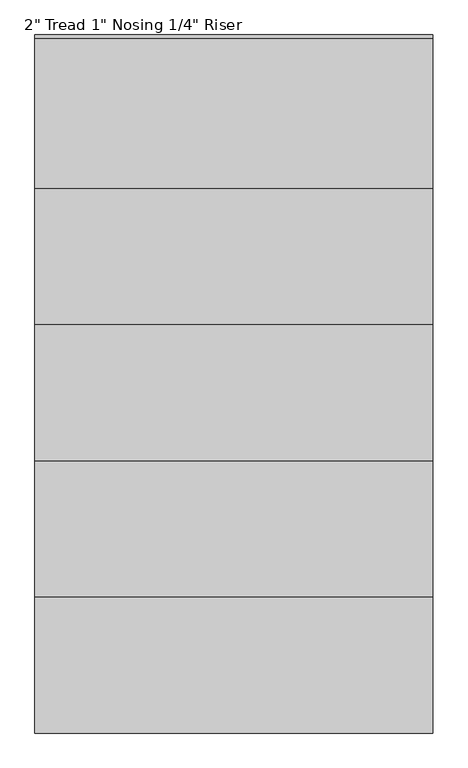
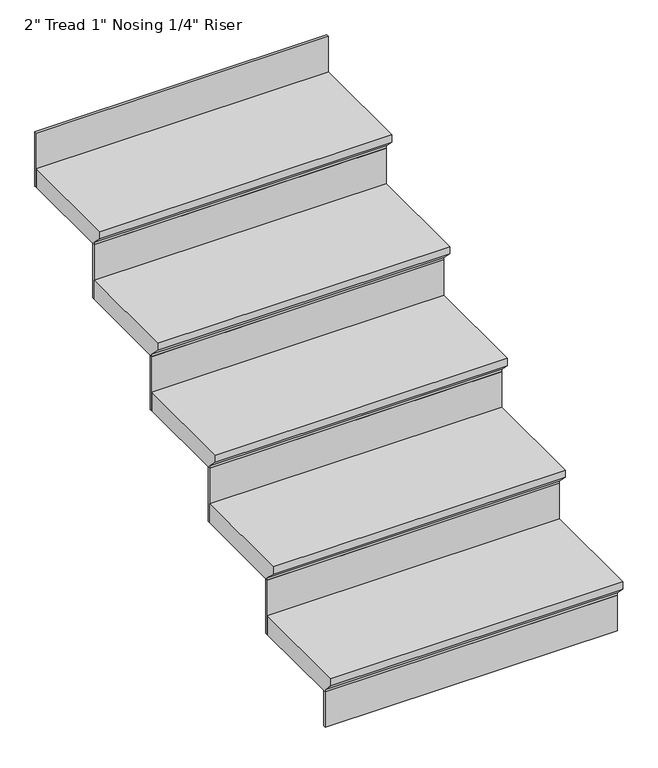
"""IFC4 building model written with IfcOpenShell, lengths in millimetres: stair flight geometry."""

from ifc_helpers import new_model, si_unit, origin, place, context, project, spatial, faceted_brep, source, transform, mapped, element, save


def stair_flight_670a0b79(model_context):
    return source(origin(), model_context, "Body", "Brep", [
        faceted_brep([(-5330.5155596, 4813.6076853, 7137.4), (-5330.5155596, 4813.6076853, 7156.45), (-6072.1955596, 4813.6076853, 7156.45), (-6072.1955596, 4813.6076853, 7137.4), (-5330.5155596, 4839.0076853, 7112.0), (-6072.1955596, 4839.0076853, 7112.0), (-5330.5155596, 5093.0076853, 7156.45), (-6072.1955596, 5093.0076853, 7156.45), (-6072.1955596, 4839.0076853, 7105.65), (-6072.1955596, 5093.0076853, 7105.65), (-5330.5155596, 5093.0076853, 7105.65), (-5330.5155596, 4839.0076853, 7105.65)], [[[0, 1, 2, 3]], [[4, 0, 3, 5]], [[2, 1, 6, 7]], [[8, 9, 10, 11]], [[2, 7, 9, 8, 5, 3]], [[8, 11, 4, 5]], [[6, 1, 0, 4, 11, 10]], [[7, 6, 10, 9]]]),
        faceted_brep([(-5330.5155596, 4839.0076853, 7105.65), (-5330.5155596, 4839.0076853, 7010.4), (-5330.5155596, 4845.3576853, 7010.4), (-5330.5155596, 4845.3576853, 7105.65), (-6072.1955596, 4839.0076853, 7105.65), (-6072.1955596, 4845.3576853, 7105.65), (-6072.1955596, 4845.3576853, 7010.4), (-6072.1955596, 4839.0076853, 7010.4)], [[[0, 1, 2, 3]], [[4, 5, 6, 7]], [[1, 0, 4, 7]], [[2, 1, 7, 6]], [[3, 2, 6, 5]], [[0, 3, 5, 4]]]),
        faceted_brep([(-5330.5155596, 5093.0076853, 7251.7), (-5330.5155596, 5093.0076853, 7105.65), (-5330.5155596, 5099.3576853, 7105.65), (-5330.5155596, 5099.3576853, 7251.7), (-6072.1955596, 5093.0076853, 7251.7), (-6072.1955596, 5099.3576853, 7251.7), (-6072.1955596, 5099.3576853, 7105.65), (-6072.1955596, 5093.0076853, 7105.65)], [[[0, 1, 2, 3]], [[4, 5, 6, 7]], [[1, 0, 4, 7]], [[2, 1, 7, 6]], [[3, 2, 6, 5]], [[0, 3, 5, 4]]]),
        faceted_brep([(-6072.1955596, 5067.6076853, 7302.5), (-5330.5155596, 5067.6076853, 7302.5), (-5330.5155596, 5347.0076853, 7302.5), (-6072.1955596, 5347.0076853, 7302.5), (-6072.1955596, 5093.0076853, 7251.7), (-6072.1955596, 5347.0076853, 7251.7), (-5330.5155596, 5347.0076853, 7251.7), (-5330.5155596, 5093.0076853, 7251.7), (-6072.1955596, 5093.0076853, 7258.05), (-6072.1955596, 5067.6076853, 7283.45), (-5330.5155596, 5093.0076853, 7258.05), (-5330.5155596, 5067.6076853, 7283.45)], [[[0, 1, 2, 3]], [[4, 5, 6, 7]], [[0, 3, 5, 4, 8, 9]], [[4, 7, 10, 8]], [[2, 1, 11, 10, 7, 6]], [[3, 2, 6, 5]], [[11, 1, 0, 9]], [[10, 11, 9, 8]]]),
        faceted_brep([(-5330.5155596, 5347.0076853, 7397.75), (-5330.5155596, 5347.0076853, 7251.7), (-5330.5155596, 5353.3576853, 7251.7), (-5330.5155596, 5353.3576853, 7397.75), (-6072.1955596, 5347.0076853, 7397.75), (-6072.1955596, 5353.3576853, 7397.75), (-6072.1955596, 5353.3576853, 7251.7), (-6072.1955596, 5347.0076853, 7251.7)], [[[0, 1, 2, 3]], [[4, 5, 6, 7]], [[1, 0, 4, 7]], [[2, 1, 7, 6]], [[3, 2, 6, 5]], [[0, 3, 5, 4]]]),
        faceted_brep([(-6072.1955596, 5321.6076853, 7448.55), (-5330.5155596, 5321.6076853, 7448.55), (-5330.5155596, 5601.0076853, 7448.55), (-6072.1955596, 5601.0076853, 7448.55), (-6072.1955596, 5347.0076853, 7397.75), (-6072.1955596, 5601.0076853, 7397.75), (-5330.5155596, 5601.0076853, 7397.75), (-5330.5155596, 5347.0076853, 7397.75), (-6072.1955596, 5347.0076853, 7404.1), (-6072.1955596, 5321.6076853, 7429.5), (-5330.5155596, 5347.0076853, 7404.1), (-5330.5155596, 5321.6076853, 7429.5)], [[[0, 1, 2, 3]], [[4, 5, 6, 7]], [[0, 3, 5, 4, 8, 9]], [[4, 7, 10, 8]], [[2, 1, 11, 10, 7, 6]], [[3, 2, 6, 5]], [[11, 1, 0, 9]], [[10, 11, 9, 8]]]),
        faceted_brep([(-5330.5155596, 5601.0076853, 7543.8), (-5330.5155596, 5601.0076853, 7397.75), (-5330.5155596, 5607.3576853, 7397.75), (-5330.5155596, 5607.3576853, 7543.8), (-6072.1955596, 5601.0076853, 7543.8), (-6072.1955596, 5607.3576853, 7543.8), (-6072.1955596, 5607.3576853, 7397.75), (-6072.1955596, 5601.0076853, 7397.75)], [[[0, 1, 2, 3]], [[4, 5, 6, 7]], [[1, 0, 4, 7]], [[2, 1, 7, 6]], [[3, 2, 6, 5]], [[0, 3, 5, 4]]]),
        faceted_brep([(-6072.1955596, 5575.6076853, 7594.6), (-5330.5155596, 5575.6076853, 7594.6), (-5330.5155596, 5855.0076853, 7594.6), (-6072.1955596, 5855.0076853, 7594.6), (-6072.1955596, 5601.0076853, 7543.8), (-6072.1955596, 5855.0076853, 7543.8), (-5330.5155596, 5855.0076853, 7543.8), (-5330.5155596, 5601.0076853, 7543.8), (-6072.1955596, 5601.0076853, 7550.15), (-6072.1955596, 5575.6076853, 7575.55), (-5330.5155596, 5601.0076853, 7550.15), (-5330.5155596, 5575.6076853, 7575.55)], [[[0, 1, 2, 3]], [[4, 5, 6, 7]], [[0, 3, 5, 4, 8, 9]], [[4, 7, 10, 8]], [[2, 1, 11, 10, 7, 6]], [[3, 2, 6, 5]], [[11, 1, 0, 9]], [[10, 11, 9, 8]]]),
        faceted_brep([(-5330.5155596, 6109.0076853, 7835.9), (-5330.5155596, 6109.0076853, 7689.85), (-5330.5155596, 6115.3576853, 7689.85), (-5330.5155596, 6115.3576853, 7835.9), (-6072.1955596, 6109.0076853, 7835.9), (-6072.1955596, 6115.3576853, 7835.9), (-6072.1955596, 6115.3576853, 7689.85), (-6072.1955596, 6109.0076853, 7689.85)], [[[0, 1, 2, 3]], [[4, 5, 6, 7]], [[1, 0, 4, 7]], [[2, 1, 7, 6]], [[3, 2, 6, 5]], [[0, 3, 5, 4]]]),
        faceted_brep([(-5330.5155596, 5855.0076853, 7689.85), (-5330.5155596, 5855.0076853, 7543.8), (-5330.5155596, 5861.3576853, 7543.8), (-5330.5155596, 5861.3576853, 7689.85), (-6072.1955596, 5855.0076853, 7689.85), (-6072.1955596, 5861.3576853, 7689.85), (-6072.1955596, 5861.3576853, 7543.8), (-6072.1955596, 5855.0076853, 7543.8)], [[[0, 1, 2, 3]], [[4, 5, 6, 7]], [[1, 0, 4, 7]], [[2, 1, 7, 6]], [[3, 2, 6, 5]], [[0, 3, 5, 4]]]),
        faceted_brep([(-6072.1955596, 5829.6076853, 7740.65), (-5330.5155596, 5829.6076853, 7740.65), (-5330.5155596, 6083.6076853, 7740.65), (-5330.5155596, 6109.0076853, 7740.65), (-6072.1955596, 6109.0076853, 7740.65), (-6072.1955596, 5855.0076853, 7689.85), (-6072.1955596, 6109.0076853, 7689.85), (-5330.5155596, 6109.0076853, 7689.85), (-5330.5155596, 6083.6076853, 7689.85), (-5330.5155596, 5855.0076853, 7689.85), (-6072.1955596, 5855.0076853, 7696.2), (-6072.1955596, 5829.6076853, 7721.6), (-5330.5155596, 5855.0076853, 7696.2), (-5330.5155596, 5829.6076853, 7721.6)], [[[0, 1, 2, 3, 4]], [[5, 6, 7, 8, 9]], [[0, 4, 6, 5, 10, 11]], [[5, 9, 12, 10]], [[2, 1, 13, 12, 9, 8]], [[3, 2, 8, 7]], [[4, 3, 7, 6]], [[13, 1, 0, 11]], [[12, 13, 11, 10]]]),
    ])


if __name__ == "__main__":
    model = new_model("IFC4")
    model_context = context("Model", 3, world=origin())
    ifc_project = project(units=[si_unit("LENGTHUNIT", "METRE", prefix="MILLI")], contexts=[model_context])
    site = spatial("IfcSite", under=ifc_project)
    building = spatial("IfcBuilding", under=site)
    placement = place(None, origin())
    stair_flight_shape = stair_flight_670a0b79(model_context)
    element("IfcStairFlight", 1, ObjectType="2\" Tread 1\" Nosing 1/4\" Riser", at=placement, inside=building, context=model_context, shape_type="MappedRepresentation", body=[
        mapped(stair_flight_shape, transform((0.0, 0.0, 0.0), x_axis=(1.0, 0.0, 0.0), y_axis=(0.0, 1.0, 0.0), z_axis=(0.0, 0.0, 1.0))),
    ])
    save(model, "model.ifc")
